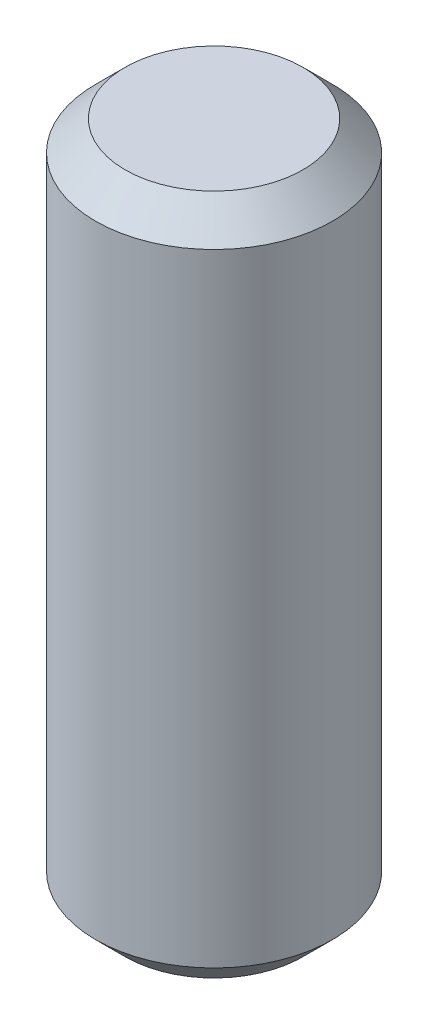
from build123d import *

# Parameters (mm, degrees)
PIN_PROFILE_4_R           = 2
PIN_BODY_4X18_DEPTH       = 11.5
END_CHAMFER_A_0_5X45_SIZE = 0.5
END_CHAMFER_B_0_5X45_SIZE = 0.5


with BuildPart() as part:
    # Pin Profile Ø4 → Pin Body Ø4x18 (new body)
    with BuildSketch(Plane(origin=(0, 0, 0), x_dir=(1, 0, 0), z_dir=(0, 1, 0))):
        with Locations(Location((0, 0, 0), (0, 0, 270))):
            Circle(PIN_PROFILE_4_R)
    extrude(amount=PIN_BODY_4X18_DEPTH)

    # End Chamfer A 0.5x45°
    end_chamfer_a_0_5x45_edges = [part.edges().sort_by_distance(p)[0] for p in [
        (0, 11.5, -2),
    ]]
    chamfer(end_chamfer_a_0_5x45_edges, length=END_CHAMFER_A_0_5X45_SIZE)

    # End Chamfer B 0.5x45°
    end_chamfer_b_0_5x45_edges = [part.edges().sort_by_distance(p)[0] for p in [
        (0, 0, -2),
    ]]
    chamfer(end_chamfer_b_0_5x45_edges, length=END_CHAMFER_B_0_5X45_SIZE)


solid = part.part
